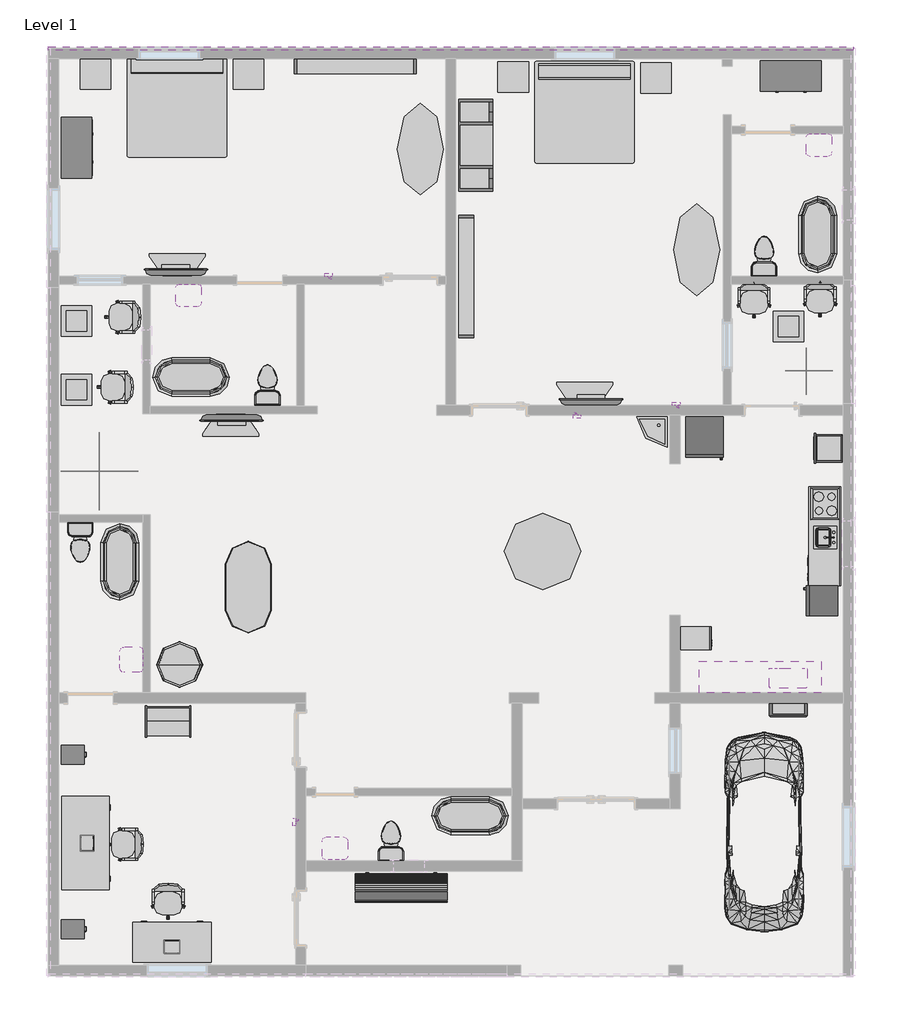
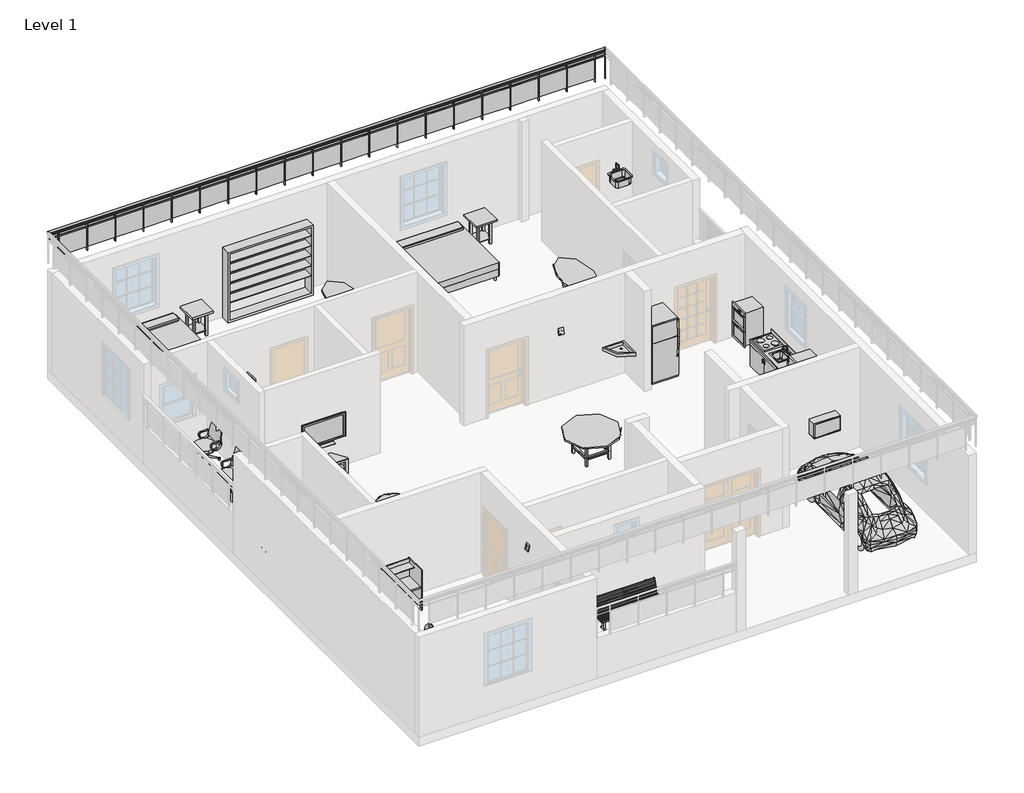
# One storey, part 4 of 4: 37 furniture elements, 17 proxies, 14 flow terminals, 3 geographic elements, 1 railing.
"""IFC4 building model written with IfcOpenShell, lengths in millimetres."""

from ifc_helpers import new_model, si_unit, point, frame, origin, place, context, project, spatial, polyline, ellipse_curve, trimmed, outline, extrude, transform, mapped, element, save
from ifc_brep_helpers import plane_surface, extruded_surface, advanced_brep
from components import entourage_4c8cfd20, proxy_7e1014cc, proxy_a6faaae8, proxy_45b28599, kitchenette_medium_kitchenette_medium_844211aa, proxy_8a8d5ab2, proxy_8b8c2dc4, rpc_beetle_rpc_beetle_3ce7ba48, rpc_picture_frame_rpc_picture_frame_c25e3fe9, proxy_c523a7b7, proxy_a13a33b2, single_carrel_single_carrel_ed4d160c, flow_terminal_bd5cdcf8, flow_terminal_871c2e40, flow_terminal_62a433f7, toilet_domestic_3d_toilet_domestic_3d_f7549cf7, toilet_domestic_3d_toilet_domestic_3d_183bbd19, flow_terminal_b374fae2, furniture_1fc5af50, furniture_d4d3357e, chair_executive_chair_executive_8d69e98c, furniture_22cae41e, furniture_c6510c7c, furniture_072f6425, furniture_2fc54265, furniture_9fa109b2, furniture_cf0b6580, furniture_b1da5ad0, furniture_fdf74506, tv_stand_tv_stand_6ce107e5, furniture_b5c51a22, furniture_2c34a4f9, furniture_bbcc68ce, furniture_027a2ad9, furniture_5bc9ed15, furniture_c80d6d9c, geographic_element_235d1464, geographic_element_ca6e1e19, geographic_element_e27c54a3

model = new_model("IFC4")

# Units and contexts
model_context = context("Model", 3, world=origin())
ifc_project = project(units=[si_unit("LENGTHUNIT", "METRE", prefix="MILLI")], contexts=[model_context])

# Site, building, storey
site = spatial("IfcSite", under=ifc_project)
building = spatial("IfcBuilding", under=site)
storey = spatial("IfcBuildingStorey", under=building, Name="Level 1", Elevation=0.0)

# Proxies
placement = place(None, origin())
entourage_shape = entourage_4c8cfd20(model_context)
element("IfcBuildingElementProxy", 1, Name="Entourage", at=placement, inside=storey, context=model_context, shape_type="MappedRepresentation", body=[
    mapped(entourage_shape, transform((-16905.1484731, -3276.9557719, 762.0), x_axis=(0.0, 1.0, 0.0), y_axis=(-1.0, 0.0, 0.0), z_axis=(0.0, 0.0, 1.0))),
])
element("IfcBuildingElementProxy", 2, Name="Entourage", at=placement, inside=storey, context=model_context, shape_type="MappedRepresentation", body=[
    mapped(entourage_shape, transform((-15177.9484731, -5385.1557719, 762.0), x_axis=(-1.0, 0.0, 0.0), y_axis=(0.0, -1.0, 0.0), z_axis=(0.0, 0.0, 1.0))),
])
proxy_shape = proxy_7e1014cc(model_context)
element("IfcBuildingElementProxy", 3, Name="18\" x 24\" x 34 1/2\"", ObjectType="18\" x 24\" x 34 1/2\"", at=placement, inside=storey, context=model_context, shape_type="MappedRepresentation", body=[
    mapped(proxy_shape, transform((-4472.0989083, 506.3267596, 0.0), x_axis=(0.0, 1.0, 0.0), y_axis=(-1.0, 0.0, 0.0), z_axis=(0.0, 0.0, 1.0))),
])
proxy_2_shape = proxy_a6faaae8(model_context)
element("IfcBuildingElementProxy", 4, Name="Cook Top-4 Unit2 : 22\" x 20\"", ObjectType="Cook Top-4 Unit2 : 22\" x 20\"", at=placement, inside=storey, context=model_context, shape_type="MappedRepresentation", body=[
    mapped(proxy_2_shape, transform((-2147.7484731, 3492.1442281, 0.0), x_axis=(0.0, -1.0, 0.0), y_axis=(1.0, 0.0, 0.0), z_axis=(0.0, 0.0, 1.0))),
])
proxy_3_shape = proxy_45b28599(model_context)
element("IfcBuildingElementProxy", 5, Name="Dishwasher : 24\" x 24\" x 34\"", ObjectType="Dishwasher : 24\" x 24\" x 34\"", at=placement, inside=storey, context=model_context, shape_type="MappedRepresentation", body=[
    mapped(proxy_3_shape, transform((-2439.5980379, 2540.9616966, 0.0), x_axis=(0.0, -1.0, 0.0), y_axis=(1.0, 0.0, 0.0), z_axis=(0.0, 0.0, 1.0))),
])
kitchenette_medium_kitchenette_medium_shape = kitchenette_medium_kitchenette_medium_844211aa(model_context)
element("IfcBuildingElementProxy", 6, Name="Kitchenette - Medium : Kitchenette - Medium", ObjectType="Kitchenette - Medium : Kitchenette - Medium", at=placement, inside=storey, context=model_context, shape_type="MappedRepresentation", body=[
    mapped(kitchenette_medium_kitchenette_medium_shape, transform((-1842.9484731, 3167.981933, 0.0), x_axis=(0.0, -1.0, 0.0), y_axis=(1.0, 0.0, 0.0), z_axis=(0.0, 0.0, 1.0))),
])
proxy_4_shape = proxy_8a8d5ab2(model_context)
element("IfcBuildingElementProxy", 7, Name="Microwave : 30\" x 16\" x 18\"", ObjectType="Microwave : 30\" x 16\" x 18\"", at=placement, inside=storey, context=model_context, shape_type="MappedRepresentation", body=[
    mapped(proxy_4_shape, transform((-2384.0555957, -912.2362777, 0.0), x_axis=(-1.0000000000000004, 0.0, 0.0), y_axis=(0.0, -1.0000000000000004, 0.0), z_axis=(0.0, 0.0, 1.0))),
])
element("IfcBuildingElementProxy", 8, Name="Microwave : 30\" x 16\" x 18\"", ObjectType="Microwave : 30\" x 16\" x 18\"", at=placement, inside=storey, context=model_context, shape_type="MappedRepresentation", body=[
    mapped(proxy_4_shape, transform((-2384.0555957, -340.7362777, 609.6), x_axis=(-1.0000000000000013, 0.0, 0.0), y_axis=(0.0, -1.0000000000000013, 0.0), z_axis=(0.0, 0.0, 1.0))),
])
proxy_5_shape = proxy_8b8c2dc4(model_context)
element("IfcBuildingElementProxy", 9, Name="Oven Double-Built-in : 21 1/2\" x 39 1/4\" x 21\"", ObjectType="Oven Double-Built-in : 21 1/2\" x 39 1/4\" x 21\"", at=placement, inside=storey, context=model_context, shape_type="MappedRepresentation", body=[
    mapped(proxy_5_shape, transform((-2212.614332, 4561.8693008, 0.0), x_axis=(0.0, -1.0000000000000004, 0.0), y_axis=(1.0000000000000004, 0.0, 0.0), z_axis=(0.0, 0.0, 1.0))),
])
rpc_beetle_rpc_beetle_shape = rpc_beetle_rpc_beetle_3ce7ba48(model_context)
element("IfcBuildingElementProxy", 10, Name="RPC Beetle : RPC Beetle", ObjectType="RPC Beetle : RPC Beetle", at=placement, inside=storey, context=model_context, shape_type="MappedRepresentation", body=[
    mapped(rpc_beetle_rpc_beetle_shape, transform((-3366.9484731, -4292.9557719, 0.0), x_axis=(1.0, 0.0, 0.0), y_axis=(0.0, 1.0, 0.0), z_axis=(0.0, 0.0, 1.0))),
])
rpc_picture_frame_rpc_picture_frame_shape = rpc_picture_frame_rpc_picture_frame_c25e3fe9(model_context)
element("IfcBuildingElementProxy", 11, Name="RPC Picture Frame : RPC Picture Frame", ObjectType="RPC Picture Frame : RPC Picture Frame", at=placement, inside=storey, context=model_context, shape_type="MappedRepresentation", body=[
    mapped(rpc_picture_frame_rpc_picture_frame_shape, transform((-12053.7484731, 8026.0442281, 1828.8), x_axis=(-1.0000000000000002, 0.0, 0.0), y_axis=(0.0, -1.0000000000000002, 0.0), z_axis=(0.0, 0.0, 1.0))),
])
element("IfcBuildingElementProxy", 12, Name="RPC Picture Frame : RPC Picture Frame", ObjectType="RPC Picture Frame : RPC Picture Frame", at=placement, inside=storey, context=model_context, shape_type="MappedRepresentation", body=[
    mapped(rpc_picture_frame_rpc_picture_frame_shape, transform((-5119.5484731, 5460.6442281, 1828.8), x_axis=(-1.0000000000000002, 0.0, 0.0), y_axis=(0.0, -1.0000000000000002, 0.0), z_axis=(0.0, 0.0, 1.0))),
])
element("IfcBuildingElementProxy", 13, Name="RPC Picture Frame : RPC Picture Frame", ObjectType="RPC Picture Frame : RPC Picture Frame", at=placement, inside=storey, context=model_context, shape_type="MappedRepresentation", body=[
    mapped(rpc_picture_frame_rpc_picture_frame_shape, transform((-7100.7484731, 5257.4442281, 1828.8), x_axis=(1.0, 0.0, 0.0), y_axis=(0.0, 1.0, 0.0), z_axis=(0.0, 0.0, 1.0))),
])
element("IfcBuildingElementProxy", 14, Name="RPC Picture Frame : RPC Picture Frame", ObjectType="RPC Picture Frame : RPC Picture Frame", at=placement, inside=storey, context=model_context, shape_type="MappedRepresentation", body=[
    mapped(rpc_picture_frame_rpc_picture_frame_shape, transform((-12714.1484731, -2857.8557719, 2133.6), x_axis=(0.0, -1.0, 0.0), y_axis=(1.0, 0.0, 0.0), z_axis=(0.0, 0.0, 1.0))),
])
proxy_6_shape = proxy_c523a7b7(model_context)
element("IfcBuildingElementProxy", 15, Name="Refrigerator : 24\" x 25\" LH", ObjectType="Refrigerator : 24\" x 25\" LH", at=placement, inside=storey, context=model_context, shape_type="MappedRepresentation", body=[
    mapped(proxy_6_shape, transform((-2193.3974446, 1555.3942281, 0.0), x_axis=(0.0, -1.0, 0.0), y_axis=(1.0, 0.0, 0.0), z_axis=(0.0, 0.0, 1.0))),
])
proxy_7_shape = proxy_a13a33b2(model_context)
element("IfcBuildingElementProxy", 16, Name="Refrigerator.0001 : 30\" x 32\" RH", ObjectType="Refrigerator.0001 : 30\" x 32\" RH", at=placement, inside=storey, context=model_context, shape_type="MappedRepresentation", body=[
    mapped(proxy_7_shape, transform((-4552.8109731, 4839.5431996, 0.0), x_axis=(1.0000000000000009, 0.0, 0.0), y_axis=(0.0, 1.0000000000000009, 0.0), z_axis=(0.0, 0.0, 1.0))),
])
single_carrel_single_carrel_shape = single_carrel_single_carrel_ed4d160c(model_context)
element("IfcBuildingElementProxy", 17, Name="Single Carrel : Single Carrel", ObjectType="Single Carrel : Single Carrel", at=placement, inside=storey, context=model_context, shape_type="MappedRepresentation", body=[
    mapped(single_carrel_single_carrel_shape, transform((-15254.1484731, -559.1557719, 0.0), x_axis=(1.0, 0.0, 0.0), y_axis=(0.0, 1.0, 0.0), z_axis=(0.0, 0.0, 1.0))),
])

# Flow terminals
flow_terminal_shape = flow_terminal_bd5cdcf8(model_context)
element("IfcFlowTerminal", 18, ObjectType="Sink - Corner Floor : 24\"", at=placement, inside=storey, context=model_context, shape_type="MappedRepresentation", body=[
    mapped(flow_terminal_shape, transform((-5297.3484731, 5232.0442281, 914.4), x_axis=(-1.0000000000000002, 0.0, 0.0), y_axis=(0.0, -1.0000000000000002, 0.0), z_axis=(0.0, 0.0, 1.0))),
])
flow_terminal_2_shape = flow_terminal_871c2e40(model_context)
element("IfcFlowTerminal", 19, ObjectType="Sink Kitchen-Island : 18\" x 18\"", at=placement, inside=storey, context=model_context, shape_type="MappedRepresentation", body=[
    mapped(flow_terminal_2_shape, transform((-2150.0938742, 2834.7334687, -14.4), x_axis=(0.0, -1.0, 0.0), y_axis=(1.0, 0.0, 0.0), z_axis=(0.0, 0.0, 1.0))),
])
flow_terminal_3_shape = flow_terminal_62a433f7(model_context)
element("IfcFlowTerminal", 20, ObjectType="Sink Vanity-Square : 20\" x 18\"", at=placement, inside=storey, context=model_context, shape_type="MappedRepresentation", body=[
    mapped(flow_terminal_3_shape, transform((-14863.4377136, 7693.498827, 914.4), x_axis=(1.0, 0.0, 0.0), y_axis=(0.0, 1.0, 0.0), z_axis=(0.0, 0.0, 1.0))),
])
element("IfcFlowTerminal", 21, ObjectType="Sink Vanity-Square : 20\" x 18\"", at=placement, inside=storey, context=model_context, shape_type="MappedRepresentation", body=[
    mapped(flow_terminal_3_shape, transform((-2290.4377136, 10690.698827, 914.4), x_axis=(1.0, 0.0, 0.0), y_axis=(0.0, 1.0, 0.0), z_axis=(0.0, 0.0, 1.0))),
])
element("IfcFlowTerminal", 22, ObjectType="Sink Vanity-Square : 20\" x 18\"", at=placement, inside=storey, context=model_context, shape_type="MappedRepresentation", body=[
    mapped(flow_terminal_3_shape, transform((-15942.2938742, 396.3334687, 914.4), x_axis=(0.0, -1.0000000000000004, 0.0), y_axis=(1.0000000000000004, 0.0, 0.0), z_axis=(0.0, 0.0, 1.0))),
])
element("IfcFlowTerminal", 23, ObjectType="Sink Vanity-Square : 20\" x 18\"", at=placement, inside=storey, context=model_context, shape_type="MappedRepresentation", body=[
    mapped(flow_terminal_3_shape, transform((-11911.0592325, -3427.0103708, 914.4), x_axis=(-1.0, 0.0, 0.0), y_axis=(0.0, -1.0, 0.0), z_axis=(0.0, 0.0, 1.0))),
])
toilet_domestic_3d_toilet_domestic_3d_shape = toilet_domestic_3d_toilet_domestic_3d_f7549cf7(model_context)
toilet_domestic_3d_toilet_domestic_3d_2_shape = toilet_domestic_3d_toilet_domestic_3d_183bbd19(model_context)
element("IfcFlowTerminal", 24, ObjectType="Toilet-Domestic-3D : Toilet-Domestic-3D", at=placement, inside=storey, context=model_context, shape_type="MappedRepresentation", body=[
    mapped(toilet_domestic_3d_toilet_domestic_3d_shape, transform((-13272.9484731, 5955.3402555, 0.0), x_axis=(-1.0, 0.0, 0.0), y_axis=(0.0, -1.0, 0.0), z_axis=(0.0, 0.0, 1.0))),
    mapped(toilet_domestic_3d_toilet_domestic_3d_2_shape, transform((-13272.9484731, 5955.3402555, 0.0), x_axis=(-1.0, 0.0, 0.0), y_axis=(0.0, -1.0, 0.0), z_axis=(0.0, 0.0, 1.0))),
])
element("IfcFlowTerminal", 25, ObjectType="Toilet-Domestic-3D : Toilet-Domestic-3D", at=placement, inside=storey, context=model_context, shape_type="MappedRepresentation", body=[
    mapped(toilet_domestic_3d_toilet_domestic_3d_shape, transform((-3366.9484731, 8520.7402555, 0.0), x_axis=(-1.0, 0.0, 0.0), y_axis=(0.0, -1.0, 0.0), z_axis=(0.0, 0.0, 1.0))),
    mapped(toilet_domestic_3d_toilet_domestic_3d_2_shape, transform((-3366.9484731, 8520.7402555, 0.0), x_axis=(-1.0, 0.0, 0.0), y_axis=(0.0, -1.0, 0.0), z_axis=(0.0, 0.0, 1.0))),
])
element("IfcFlowTerminal", 26, ObjectType="Toilet-Domestic-3D : Toilet-Domestic-3D", at=placement, inside=storey, context=model_context, shape_type="MappedRepresentation", body=[
    mapped(toilet_domestic_3d_toilet_domestic_3d_shape, transform((-17006.7484731, 2629.1482008, 0.0), x_axis=(1.0, 0.0, 0.0), y_axis=(0.0, 1.0, 0.0), z_axis=(0.0, 0.0, 1.0))),
    mapped(toilet_domestic_3d_toilet_domestic_3d_2_shape, transform((-17006.7484731, 2629.1482008, 0.0), x_axis=(1.0, 0.0, 0.0), y_axis=(0.0, 1.0, 0.0), z_axis=(0.0, 0.0, 1.0))),
])
element("IfcFlowTerminal", 27, ObjectType="Toilet-Domestic-3D : Toilet-Domestic-3D", at=placement, inside=storey, context=model_context, shape_type="MappedRepresentation", body=[
    mapped(toilet_domestic_3d_toilet_domestic_3d_shape, transform((-10809.7524457, -3143.3728146, 0.0), x_axis=(-1.0, 0.0, 0.0), y_axis=(0.0, -1.0, 0.0), z_axis=(0.0, 0.0, 1.0))),
    mapped(toilet_domestic_3d_toilet_domestic_3d_2_shape, transform((-10809.7524457, -3143.3728146, 0.0), x_axis=(-1.0, 0.0, 0.0), y_axis=(0.0, -1.0, 0.0), z_axis=(0.0, 0.0, 1.0))),
])
flow_terminal_4_shape = flow_terminal_b374fae2(model_context)
element("IfcFlowTerminal", 28, ObjectType="Tub-Free Standing-3D : 30\" x 60\"", at=placement, inside=storey, context=model_context, shape_type="MappedRepresentation", body=[
    mapped(flow_terminal_4_shape, transform((-2300.1484731, 8864.2442281, 0.0), x_axis=(-1.0000000000000002, 0.0, 0.0), y_axis=(0.0, -1.0000000000000002, 0.0), z_axis=(0.0, 0.0, 1.0))),
])
element("IfcFlowTerminal", 29, ObjectType="Tub-Free Standing-3D : 30\" x 60\"", at=placement, inside=storey, context=model_context, shape_type="MappedRepresentation", body=[
    mapped(flow_terminal_4_shape, transform((-14796.9484731, 6019.4442281, 0.0), x_axis=(0.0, 1.0000000000000004, 0.0), y_axis=(-1.0000000000000004, 0.0, 0.0), z_axis=(0.0, 0.0, 1.0))),
])
element("IfcFlowTerminal", 30, ObjectType="Tub-Free Standing-3D : 30\" x 60\"", at=placement, inside=storey, context=model_context, shape_type="MappedRepresentation", body=[
    mapped(flow_terminal_4_shape, transform((-16219.3484731, 2330.6431503, 0.0), x_axis=(1.0000000000000002, 0.0, 0.0), y_axis=(0.0, 1.0000000000000002, 0.0), z_axis=(0.0, 0.0, 1.0))),
])
element("IfcFlowTerminal", 31, ObjectType="Tub-Free Standing-3D : 30\" x 60\"", at=placement, inside=storey, context=model_context, shape_type="MappedRepresentation", body=[
    mapped(flow_terminal_4_shape, transform((-9234.3484731, -2733.7411816, 0.0), x_axis=(0.0, -1.0000000000000004, 0.0), y_axis=(1.0000000000000004, 0.0, 0.0), z_axis=(0.0, 0.0, 1.0))),
])

# Furniture
furniture_shape = furniture_1fc5af50(model_context)
element("IfcFurniture", 32, ObjectType="Bed-Standard.0001 : King 78\" x 80\"", at=placement, inside=storey, context=model_context, shape_type="MappedRepresentation", body=[
    mapped(furniture_shape, transform((-15347.8369977, 11462.5393101, 0.0), x_axis=(1.0, 0.0, 0.0), y_axis=(0.0, 1.0, 0.0), z_axis=(0.0, 0.0, 1.0))),
])
element("IfcFurniture", 33, ObjectType="Bed-Standard.0001 : King 78\" x 80\"", at=placement, inside=storey, context=model_context, shape_type="MappedRepresentation", body=[
    mapped(furniture_shape, transform((-7219.8369977, 11348.2393101, 0.0), x_axis=(1.0, 0.0, 0.0), y_axis=(0.0, 1.0, 0.0), z_axis=(0.0, 0.0, 1.0))),
])
furniture_2_shape = furniture_d4d3357e(model_context)
element("IfcFurniture", 34, ObjectType="Cabinet-File 5 Drawer : 15\" x 18\"", at=placement, inside=storey, context=model_context, shape_type="MappedRepresentation", body=[
    mapped(furniture_2_shape, transform((-17301.2827732, -4863.5593248, 0.0), x_axis=(0.0, 1.0, 0.0), y_axis=(-1.0, 0.0, 0.0), z_axis=(0.0, 0.0, 1.0))),
])
element("IfcFurniture", 35, ObjectType="Cabinet-File 5 Drawer : 15\" x 18\"", at=placement, inside=storey, context=model_context, shape_type="MappedRepresentation", body=[
    mapped(furniture_2_shape, transform((-17301.2827732, -1383.7593248, 0.0), x_axis=(0.0, 1.0, 0.0), y_axis=(-1.0, 0.0, 0.0), z_axis=(0.0, 0.0, 1.0))),
])
chair_executive_chair_executive_shape = chair_executive_chair_executive_8d69e98c(model_context)
element("IfcFurniture", 36, ObjectType="Chair-Executive : Chair-Executive", at=placement, inside=storey, context=model_context, shape_type="MappedRepresentation", body=[
    mapped(chair_executive_chair_executive_shape, transform((-16149.6025714, 7072.2534084, 0.0), x_axis=(0.0, 1.0, 0.0), y_axis=(-1.0, 0.0, 0.0), z_axis=(0.0, 0.0, 1.0))),
])
element("IfcFurniture", 37, ObjectType="Chair-Executive : Chair-Executive", at=placement, inside=storey, context=model_context, shape_type="MappedRepresentation", body=[
    mapped(chair_executive_chair_executive_shape, transform((-16302.0025714, 5675.2534084, 0.0), x_axis=(0.0, 1.0, 0.0), y_axis=(-1.0, 0.0, 0.0), z_axis=(0.0, 0.0, 1.0))),
])
element("IfcFurniture", 38, ObjectType="Chair-Executive : Chair-Executive", at=placement, inside=storey, context=model_context, shape_type="MappedRepresentation", body=[
    mapped(chair_executive_chair_executive_shape, transform((-3429.1576534, 7562.3901298, 0.0), x_axis=(-1.0000000000000018, 0.0, 0.0), y_axis=(0.0, -1.0000000000000018, 0.0), z_axis=(0.0, 0.0, 1.0))),
])
element("IfcFurniture", 39, ObjectType="Chair-Executive : Chair-Executive", at=placement, inside=storey, context=model_context, shape_type="MappedRepresentation", body=[
    mapped(chair_executive_chair_executive_shape, transform((-2108.3576534, 7587.7901298, 0.0), x_axis=(-1.0000000000000002, 0.0, 0.0), y_axis=(0.0, -1.0000000000000002, 0.0), z_axis=(0.0, 0.0, 1.0))),
])
element("IfcFurniture", 40, ObjectType="Chair-Executive : Chair-Executive", at=placement, inside=storey, context=model_context, shape_type="MappedRepresentation", body=[
    mapped(chair_executive_chair_executive_shape, transform((-16098.8025714, -3443.3465916, 0.0), x_axis=(0.0, 1.0, 0.0), y_axis=(-1.0, 0.0, 0.0), z_axis=(0.0, 0.0, 1.0))),
])
element("IfcFurniture", 41, ObjectType="Chair-Executive : Chair-Executive", at=placement, inside=storey, context=model_context, shape_type="MappedRepresentation", body=[
    mapped(chair_executive_chair_executive_shape, transform((-15113.1576534, -4426.4098702, 0.0), x_axis=(-1.0000000000000002, 0.0, 0.0), y_axis=(0.0, -1.0000000000000002, 0.0), z_axis=(0.0, 0.0, 1.0))),
])
furniture_3_shape = furniture_22cae41e(model_context)
element("IfcFurniture", 42, ObjectType="Counter Top w Sink Hole : 24\" Depth", at=placement, inside=storey, context=model_context, shape_type="MappedRepresentation", body=[
    mapped(furniture_3_shape, transform((-3461.886178, 355.2442281, 609.6), x_axis=(1.0, 0.0, 0.0), y_axis=(0.0, 1.0, 0.0), z_axis=(0.0, 0.0, 1.0))),
])
furniture_4_shape = furniture_c6510c7c(model_context)
element("IfcFurniture", 43, ObjectType="Counter Top w Sink Hole : 24\" Depth", at=placement, inside=storey, context=model_context, shape_type="MappedRepresentation", body=[
    mapped(furniture_4_shape, transform((-1842.9484731, 2634.581933, -14.4), x_axis=(0.0, -1.0, 0.0), y_axis=(1.0, 0.0, 0.0), z_axis=(0.0, 0.0, 1.0))),
])
furniture_5_shape = furniture_072f6425(model_context)
element("IfcFurniture", 44, ObjectType="Desk : 60\" x 30\" Student", at=placement, inside=storey, context=model_context, shape_type="MappedRepresentation", body=[
    mapped(furniture_5_shape, transform((-15939.9484731, -5639.1557719, 0.0), x_axis=(1.0, 0.0, 0.0), y_axis=(0.0, 1.0, 0.0), z_axis=(0.0, 0.0, 1.0))),
])
furniture_6_shape = furniture_2fc54265(model_context)
element("IfcFurniture", 45, ObjectType="Desk : 72\" x 36\"", at=placement, inside=storey, context=model_context, shape_type="MappedRepresentation", body=[
    mapped(furniture_6_shape, transform((-17362.3484731, -2362.5557719, 0.0), x_axis=(0.0, -1.0000000000000004, 0.0), y_axis=(1.0000000000000004, 0.0, 0.0), z_axis=(0.0, 0.0, 1.0))),
])
furniture_7_shape = furniture_9fa109b2(model_context)
element("IfcFurniture", 46, ObjectType="Dresser : 48\" x 72\" x 24\"", at=placement, inside=storey, context=model_context, shape_type="MappedRepresentation", body=[
    mapped(furniture_7_shape, transform((-17446.1114272, 10860.637488, 0.0), x_axis=(0.0, 1.0, 0.0), y_axis=(-1.0, 0.0, 0.0), z_axis=(0.0, 0.0, 1.0))),
])
element("IfcFurniture", 47, ObjectType="Dresser : 48\" x 72\" x 24\"", at=placement, inside=storey, context=model_context, shape_type="MappedRepresentation", body=[
    mapped(furniture_7_shape, transform((-2564.3552132, 12389.7071822, 0.0), x_axis=(1.0000000000000007, 0.0, 0.0), y_axis=(0.0, 1.0000000000000007, 0.0), z_axis=(0.0, 0.0, 1.0))),
])
furniture_8_shape = furniture_cf0b6580(model_context)
element("IfcFurniture", 48, ObjectType="Entertainment Center : 72\" x 72\" x 24\"", at=placement, inside=storey, context=model_context, shape_type="MappedRepresentation", body=[
    mapped(furniture_8_shape, transform((-9564.5484731, 10642.2442281, 0.0), x_axis=(0.0, 1.0, 0.0), y_axis=(-1.0, 0.0, 0.0), z_axis=(0.0, 0.0, 1.0))),
])
furniture_9_shape = furniture_b1da5ad0(model_context)
element("IfcFurniture", 49, ObjectType="Shelving : 96\" x 12\" x 84\"", at=placement, inside=storey, context=model_context, shape_type="MappedRepresentation", body=[
    mapped(furniture_9_shape, transform((-11520.3484731, 12521.8442281, 0.0), x_axis=(1.0, 0.0, 0.0), y_axis=(0.0, 1.0, 0.0), z_axis=(0.0, 0.0, 1.0))),
])
element("IfcFurniture", 50, ObjectType="Shelving : 96\" x 12\" x 84\"", at=placement, inside=storey, context=model_context, shape_type="MappedRepresentation", body=[
    mapped(furniture_9_shape, transform((-9615.3484731, 8026.0442281, 0.0), x_axis=(0.0, 1.0000000000000002, 0.0), y_axis=(-1.0000000000000002, 0.0, 0.0), z_axis=(0.0, 0.0, 1.0))),
])
furniture_10_shape = furniture_fdf74506(model_context)
element("IfcFurniture", 51, ObjectType="TV - Flat Screen : 50\"", at=placement, inside=storey, context=model_context, shape_type="MappedRepresentation", body=[
    mapped(furniture_10_shape, transform((-15105.6929872, 8105.4337019, 914.4), x_axis=(-1.0000000000000002, 0.0, 0.0), y_axis=(0.0, -1.0000000000000002, 0.0), z_axis=(0.0, 0.0, 1.0))),
])
element("IfcFurniture", 52, ObjectType="TV - Flat Screen : 50\"", at=placement, inside=storey, context=model_context, shape_type="MappedRepresentation", body=[
    mapped(furniture_10_shape, transform((-6825.2929872, 5519.1828518, 914.4), x_axis=(-1.0000000000000002, 0.0, 0.0), y_axis=(0.0, -1.0000000000000002, 0.0), z_axis=(0.0, 0.0, 1.0))),
])
element("IfcFurniture", 53, ObjectType="TV - Flat Screen : 50\"", at=placement, inside=storey, context=model_context, shape_type="MappedRepresentation", body=[
    mapped(furniture_10_shape, transform((-13982.5656994, 5210.6304677, 914.4), x_axis=(1.0000000000000007, 0.0, 0.0), y_axis=(0.0, 1.0000000000000007, 0.0), z_axis=(0.0, 0.0, 1.0))),
])
tv_stand_tv_stand_shape = tv_stand_tv_stand_6ce107e5(model_context)
element("IfcFurniture", 54, ObjectType="TV Stand : TV Stand", at=placement, inside=storey, context=model_context, shape_type="MappedRepresentation", body=[
    mapped(tv_stand_tv_stand_shape, transform((-14951.160471, 8026.0442281, 0.0), x_axis=(-1.0, 0.0, 0.0), y_axis=(0.0, -1.0, 0.0), z_axis=(0.0, 0.0, 1.0))),
])
element("IfcFurniture", 55, ObjectType="TV Stand : TV Stand", at=placement, inside=storey, context=model_context, shape_type="MappedRepresentation", body=[
    mapped(tv_stand_tv_stand_shape, transform((-6823.160471, 5460.6442281, 0.0), x_axis=(-1.0, 0.0, 0.0), y_axis=(0.0, -1.0, 0.0), z_axis=(0.0, 0.0, 1.0))),
])
element("IfcFurniture", 56, ObjectType="TV Stand : TV Stand", at=placement, inside=storey, context=model_context, shape_type="MappedRepresentation", body=[
    mapped(tv_stand_tv_stand_shape, transform((-14134.7364751, 5298.6986547, 0.0), x_axis=(1.0000000000000004, 0.0, 0.0), y_axis=(0.0, 1.0000000000000004, 0.0), z_axis=(0.0, 0.0, 1.0))),
])
furniture_11_shape = furniture_b5c51a22(model_context)
element("IfcFurniture", 57, ObjectType="Table-Coffee : 24\" x 24\" x 24\"", at=placement, inside=storey, context=model_context, shape_type="MappedRepresentation", body=[
    mapped(furniture_11_shape, transform((-17101.2142397, 5670.2331503, 0.0), x_axis=(1.0, 0.0, 0.0), y_axis=(0.0, 1.0, 0.0), z_axis=(0.0, 0.0, 1.0))),
])
element("IfcFurniture", 58, ObjectType="Table-Coffee : 24\" x 24\" x 24\"", at=placement, inside=storey, context=model_context, shape_type="MappedRepresentation", body=[
    mapped(furniture_11_shape, transform((-17101.2142397, 7041.8331503, 0.0), x_axis=(1.0, 0.0, 0.0), y_axis=(0.0, 1.0, 0.0), z_axis=(0.0, 0.0, 1.0))),
])
element("IfcFurniture", 59, ObjectType="Table-Coffee : 24\" x 24\" x 24\"", at=placement, inside=storey, context=model_context, shape_type="MappedRepresentation", body=[
    mapped(furniture_11_shape, transform((-2902.6142397, 6929.6370487, 0.0), x_axis=(1.0, 0.0, 0.0), y_axis=(0.0, 1.0, 0.0), z_axis=(0.0, 0.0, 1.0))),
])
furniture_12_shape = furniture_2c34a4f9(model_context)
element("IfcFurniture", 60, ObjectType="Table-Dining Oval : 36\" x 72\"", at=placement, inside=storey, context=model_context, shape_type="MappedRepresentation", body=[
    mapped(furniture_12_shape, transform((-14012.0468337, 2230.2639002, 0.0), x_axis=(0.0, 1.0, 0.0), y_axis=(-1.0, 0.0, 0.0), z_axis=(0.0, 0.0, 1.0))),
])
furniture_13_shape = furniture_bbcc68ce(model_context)
element("IfcFurniture", 61, ObjectType="Table-Dining Round w Chairs : 60\" Diameter", at=placement, inside=storey, context=model_context, shape_type="MappedRepresentation", body=[
    mapped(furniture_13_shape, transform((-7890.2304403, 2724.5229166, 0.0), x_axis=(1.0, 0.0, 0.0), y_axis=(0.0, 1.0, 0.0), z_axis=(0.0, 0.0, 1.0))),
])
furniture_14_shape = furniture_027a2ad9(model_context)
element("IfcFurniture", 62, ObjectType="Table-Ellipse : 72\" x 36\"", at=placement, inside=storey, context=model_context, shape_type="MappedRepresentation", body=[
    mapped(furniture_14_shape, transform((-10224.9484731, 10566.0442281, 0.0), x_axis=(0.0, 1.0, 0.0), y_axis=(-1.0, 0.0, 0.0), z_axis=(0.0, 0.0, 1.0))),
])
element("IfcFurniture", 63, ObjectType="Table-Ellipse : 72\" x 36\"", at=placement, inside=storey, context=model_context, shape_type="MappedRepresentation", body=[
    mapped(furniture_14_shape, transform((-4713.1484731, 8559.4442281, 0.0), x_axis=(0.0, -1.0000000000000007, 0.0), y_axis=(1.0000000000000007, 0.0, 0.0), z_axis=(0.0, 0.0, 1.0))),
])
furniture_15_shape = furniture_5bc9ed15(model_context)
element("IfcFurniture", 64, ObjectType="Table-Night Stand : 24\" x 24\" x 30\"", at=placement, inside=storey, context=model_context, shape_type="MappedRepresentation", body=[
    mapped(furniture_15_shape, transform((-17010.4821034, 11759.8442281, 0.0), x_axis=(1.0, 0.0, 0.0), y_axis=(0.0, 1.0, 0.0), z_axis=(0.0, 0.0, 1.0))),
])
element("IfcFurniture", 65, ObjectType="Table-Night Stand : 24\" x 24\" x 30\"", at=placement, inside=storey, context=model_context, shape_type="MappedRepresentation", body=[
    mapped(furniture_15_shape, transform((-13962.4821034, 11759.8442281, 0.0), x_axis=(1.0, 0.0, 0.0), y_axis=(0.0, 1.0, 0.0), z_axis=(0.0, 0.0, 1.0))),
])
element("IfcFurniture", 66, ObjectType="Table-Night Stand : 24\" x 24\" x 30\"", at=placement, inside=storey, context=model_context, shape_type="MappedRepresentation", body=[
    mapped(furniture_15_shape, transform((-8679.2821034, 11695.4815518, 0.0), x_axis=(1.0, 0.0, 0.0), y_axis=(0.0, 1.0, 0.0), z_axis=(0.0, 0.0, 1.0))),
])
element("IfcFurniture", 67, ObjectType="Table-Night Stand : 24\" x 24\" x 30\"", at=placement, inside=storey, context=model_context, shape_type="MappedRepresentation", body=[
    mapped(furniture_15_shape, transform((-5834.4821034, 11675.6602635, 0.0), x_axis=(1.0, 0.0, 0.0), y_axis=(0.0, 1.0, 0.0), z_axis=(0.0, 0.0, 1.0))),
])
furniture_16_shape = furniture_c80d6d9c(model_context)
element("IfcFurniture", 68, ObjectType="Table-Round : 36\" Diameter", at=placement, inside=storey, context=model_context, shape_type="MappedRepresentation", body=[
    mapped(furniture_16_shape, transform((-15025.5484731, 285.3942281, 0.0), x_axis=(1.0, 0.0, 0.0), y_axis=(0.0, 1.0, 0.0), z_axis=(0.0, 0.0, 1.0))),
])

# Geographic elements
geographic_element_shape = geographic_element_235d1464(model_context)
element("IfcGeographicElement", 69, ObjectType="Park Bench : 72\"", at=placement, inside=storey, context=model_context, shape_type="MappedRepresentation", body=[
    mapped(geographic_element_shape, transform((-10605.9484731, -4140.5557719, 0.0), x_axis=(1.0, 0.0, 0.0), y_axis=(0.0, 1.0, 0.0), z_axis=(0.0, 0.0, 1.0))),
])
geographic_element_2_shape = geographic_element_ca6e1e19(model_context)
element("IfcGeographicElement", 70, ObjectType="RPC Shrub : Burning Bush 4'-6\"", at=placement, inside=storey, context=model_context, shape_type="MappedRepresentation", body=[
    mapped(geographic_element_2_shape, transform((-16625.7484731, 4139.8442281, 0.0), x_axis=(1.0, 0.0, 0.0), y_axis=(0.0, 1.0, 0.0), z_axis=(0.0, 0.0, 1.0))),
])
geographic_element_3_shape = geographic_element_e27c54a3(model_context)
element("IfcGeographicElement", 71, ObjectType="RPC Shrub : Cedar Shrub 3'-0\"", at=placement, inside=storey, context=model_context, shape_type="MappedRepresentation", body=[
    mapped(geographic_element_3_shape, transform((-2528.7484731, 6146.4442281, 0.0), x_axis=(1.0, 0.0, 0.0), y_axis=(0.0, 1.0, 0.0), z_axis=(0.0, 0.0, 1.0))),
])

# Railing
element("IfcRailing", 72, ObjectType="Glass Panel - Bottom Fill", at=placement, inside=storey, context=model_context, shape_type="SolidModel", body=[
    advanced_brep(
    [(-17641.7484731, 12610.7442281, 4165.6), (-17641.7484731, 12534.5442281, 4165.6), (-1588.9484731, 12610.7442281, 4165.6), (-1588.9484731, 12534.5442281, 4165.6)],
    [
        (0, 1, ellipse_curve(frame((-17641.7484731, 12572.6442281, 4165.6), z_axis=(-1.0, 0.0, 0.0), x_axis=(0.0, -1.0, 0.0)), 38.1, 28.575)),
        (1, 0, ellipse_curve(frame((-17641.7484731, 12572.6442281, 4165.6), z_axis=(-1.0, 0.0, 0.0), x_axis=(0.0, -1.0, 0.0)), 38.1, 28.575)),
        (2, 3, ellipse_curve(frame((-1588.9484731, 12572.6442281, 4165.6), z_axis=(1.0, 0.0, 0.0), x_axis=(0.0, -1.0, 0.0)), 38.1, 28.575)),
        (3, 2, ellipse_curve(frame((-1588.9484731, 12572.6442281, 4165.6), z_axis=(1.0, 0.0, 0.0), x_axis=(0.0, -1.0, 0.0)), 38.1, 28.575)),
        (0, 2),
        (3, 1),
    ],
    [
        plane_surface(frame((-17641.7484731, 12572.6442281, 4165.6), z_axis=(-1.0, 0.0, 0.0), x_axis=(0.0, 1.0, 0.0))),
        plane_surface(frame((-1588.9484731, 12572.6442281, 4165.6), z_axis=(1.0, 0.0, 0.0), x_axis=(0.0, 1.0, 0.0))),
        extruded_surface(trimmed(ellipse_curve(frame((-1588.9484731, 12572.6442281, 4165.6), z_axis=(-1.0, 0.0, 0.0), x_axis=(0.0, -1.0, 0.0)), 38.1, 28.575), [point((-1588.9484731, 12610.7442281, 4165.6))], [point((-1588.9484731, 12534.5442281, 4165.6))], True, "CARTESIAN"), (-16052.800000000001, 0.0, 0.0), 16052.800000000001),
        extruded_surface(trimmed(ellipse_curve(frame((-1588.9484731, 12572.6442281, 4165.6), z_axis=(-1.0, 0.0, 0.0), x_axis=(0.0, -1.0, 0.0)), 38.1, 28.575), [point((-1588.9484731, 12534.5442281, 4165.6))], [point((-1588.9484731, 12610.7442281, 4165.6))], True, "CARTESIAN"), (-16052.800000000001, 0.0, 0.0), 16052.800000000001),
    ],
    [
        (0, [[1, 2]]),
        (1, [[3, 4]]),
        (2, [[-1, 5, -4, 6]]),
        (3, [[-2, -6, -3, -5]]),
    ],
),
    extrude(outline(polyline([(-17641.7484731, 12559.9442281), (-17641.7484731, 12585.3442281), (-1588.9484731, 12585.3442281), (-1588.9484731, 12559.9442281), (-17641.7484731, 12559.9442281)])), frame((0.0, 0.0, 4051.3), z_axis=(0.0, 0.0, 1.0), x_axis=(1.0, 0.0, 0.0)), (0.0, 0.0, 1.0), 25.4),
    extrude(outline(polyline([(-17641.7484731, 12559.9442281), (-17641.7484731, 12585.3442281), (-1588.9484731, 12585.3442281), (-1588.9484731, 12559.9442281), (-17641.7484731, 12559.9442281)])), frame((0.0, 0.0, 3949.7), z_axis=(0.0, 0.0, 1.0), x_axis=(1.0, 0.0, 0.0)), (0.0, 0.0, 1.0), 25.4),
    extrude(outline(polyline([(-1900.0984731, 12547.2442281), (-1900.0984731, 12598.0442281), (-1887.3984731, 12598.0442281), (-1887.3984731, 12547.2442281), (-1900.0984731, 12547.2442281)])), frame((0.0, 0.0, 3251.2), z_axis=(0.0, 0.0, 1.0), x_axis=(1.0, 0.0, 0.0)), (0.0, 0.0, 1.0), 885.6788223),
    extrude(outline(polyline([(-2706.5484731, 12579.1793851), (-1893.7484731, 12579.1793851), (-1893.7484731, 12572.8293851), (-2706.5484731, 12572.8293851), (-2706.5484731, 12579.1793851)])), frame((0.0, 0.0, 3352.8), z_axis=(0.0, 0.0, 1.0), x_axis=(1.0, 0.0, 0.0)), (0.0, 0.0, 1.0), 596.9),
    extrude(outline(polyline([(-2712.8984731, 12547.2442281), (-2712.8984731, 12598.0442281), (-2700.1984731, 12598.0442281), (-2700.1984731, 12547.2442281), (-2712.8984731, 12547.2442281)])), frame((0.0, 0.0, 3251.2), z_axis=(0.0, 0.0, 1.0), x_axis=(1.0, 0.0, 0.0)), (0.0, 0.0, 1.0), 885.6788223),
    extrude(outline(polyline([(-3519.3484731, 12579.1793851), (-2706.5484731, 12579.1793851), (-2706.5484731, 12572.8293851), (-3519.3484731, 12572.8293851), (-3519.3484731, 12579.1793851)])), frame((0.0, 0.0, 3352.8), z_axis=(0.0, 0.0, 1.0), x_axis=(1.0, 0.0, 0.0)), (0.0, 0.0, 1.0), 596.9),
    extrude(outline(polyline([(-3525.6984731, 12547.2442281), (-3525.6984731, 12598.0442281), (-3512.9984731, 12598.0442281), (-3512.9984731, 12547.2442281), (-3525.6984731, 12547.2442281)])), frame((0.0, 0.0, 3251.2), z_axis=(0.0, 0.0, 1.0), x_axis=(1.0, 0.0, 0.0)), (0.0, 0.0, 1.0), 885.6788223),
    extrude(outline(polyline([(-4332.1484731, 12579.1793851), (-3519.3484731, 12579.1793851), (-3519.3484731, 12572.8293851), (-4332.1484731, 12572.8293851), (-4332.1484731, 12579.1793851)])), frame((0.0, 0.0, 3352.8), z_axis=(0.0, 0.0, 1.0), x_axis=(1.0, 0.0, 0.0)), (0.0, 0.0, 1.0), 596.9),
    extrude(outline(polyline([(-4338.4984731, 12547.2442281), (-4338.4984731, 12598.0442281), (-4325.7984731, 12598.0442281), (-4325.7984731, 12547.2442281), (-4338.4984731, 12547.2442281)])), frame((0.0, 0.0, 3251.2), z_axis=(0.0, 0.0, 1.0), x_axis=(1.0, 0.0, 0.0)), (0.0, 0.0, 1.0), 885.6788223),
    extrude(outline(polyline([(-5144.9484731, 12579.1793851), (-4332.1484731, 12579.1793851), (-4332.1484731, 12572.8293851), (-5144.9484731, 12572.8293851), (-5144.9484731, 12579.1793851)])), frame((0.0, 0.0, 3352.8), z_axis=(0.0, 0.0, 1.0), x_axis=(1.0, 0.0, 0.0)), (0.0, 0.0, 1.0), 596.9),
    extrude(outline(polyline([(-5151.2984731, 12547.2442281), (-5151.2984731, 12598.0442281), (-5138.5984731, 12598.0442281), (-5138.5984731, 12547.2442281), (-5151.2984731, 12547.2442281)])), frame((0.0, 0.0, 3251.2), z_axis=(0.0, 0.0, 1.0), x_axis=(1.0, 0.0, 0.0)), (0.0, 0.0, 1.0), 885.6788223),
    extrude(outline(polyline([(-5957.7484731, 12579.1793851), (-5144.9484731, 12579.1793851), (-5144.9484731, 12572.8293851), (-5957.7484731, 12572.8293851), (-5957.7484731, 12579.1793851)])), frame((0.0, 0.0, 3352.8), z_axis=(0.0, 0.0, 1.0), x_axis=(1.0, 0.0, 0.0)), (0.0, 0.0, 1.0), 596.9),
    extrude(outline(polyline([(-5964.0984731, 12547.2442281), (-5964.0984731, 12598.0442281), (-5951.3984731, 12598.0442281), (-5951.3984731, 12547.2442281), (-5964.0984731, 12547.2442281)])), frame((0.0, 0.0, 3251.2), z_axis=(0.0, 0.0, 1.0), x_axis=(1.0, 0.0, 0.0)), (0.0, 0.0, 1.0), 885.6788223),
    extrude(outline(polyline([(-6770.5484731, 12579.1793851), (-5957.7484731, 12579.1793851), (-5957.7484731, 12572.8293851), (-6770.5484731, 12572.8293851), (-6770.5484731, 12579.1793851)])), frame((0.0, 0.0, 3352.8), z_axis=(0.0, 0.0, 1.0), x_axis=(1.0, 0.0, 0.0)), (0.0, 0.0, 1.0), 596.9),
    extrude(outline(polyline([(-6776.8984731, 12547.2442281), (-6776.8984731, 12598.0442281), (-6764.1984731, 12598.0442281), (-6764.1984731, 12547.2442281), (-6776.8984731, 12547.2442281)])), frame((0.0, 0.0, 3251.2), z_axis=(0.0, 0.0, 1.0), x_axis=(1.0, 0.0, 0.0)), (0.0, 0.0, 1.0), 885.6788223),
    extrude(outline(polyline([(-7583.3484731, 12579.1793851), (-6770.5484731, 12579.1793851), (-6770.5484731, 12572.8293851), (-7583.3484731, 12572.8293851), (-7583.3484731, 12579.1793851)])), frame((0.0, 0.0, 3352.8), z_axis=(0.0, 0.0, 1.0), x_axis=(1.0, 0.0, 0.0)), (0.0, 0.0, 1.0), 596.9),
    extrude(outline(polyline([(-7589.6984731, 12547.2442281), (-7589.6984731, 12598.0442281), (-7576.9984731, 12598.0442281), (-7576.9984731, 12547.2442281), (-7589.6984731, 12547.2442281)])), frame((0.0, 0.0, 3251.2), z_axis=(0.0, 0.0, 1.0), x_axis=(1.0, 0.0, 0.0)), (0.0, 0.0, 1.0), 885.6788223),
    extrude(outline(polyline([(-8396.1484731, 12579.1793851), (-7583.3484731, 12579.1793851), (-7583.3484731, 12572.8293851), (-8396.1484731, 12572.8293851), (-8396.1484731, 12579.1793851)])), frame((0.0, 0.0, 3352.8), z_axis=(0.0, 0.0, 1.0), x_axis=(1.0, 0.0, 0.0)), (0.0, 0.0, 1.0), 596.9),
    extrude(outline(polyline([(-8402.4984731, 12547.2442281), (-8402.4984731, 12598.0442281), (-8389.7984731, 12598.0442281), (-8389.7984731, 12547.2442281), (-8402.4984731, 12547.2442281)])), frame((0.0, 0.0, 3251.2), z_axis=(0.0, 0.0, 1.0), x_axis=(1.0, 0.0, 0.0)), (0.0, 0.0, 1.0), 885.6788223),
    extrude(outline(polyline([(-9208.9484731, 12579.1793851), (-8396.1484731, 12579.1793851), (-8396.1484731, 12572.8293851), (-9208.9484731, 12572.8293851), (-9208.9484731, 12579.1793851)])), frame((0.0, 0.0, 3352.8), z_axis=(0.0, 0.0, 1.0), x_axis=(1.0, 0.0, 0.0)), (0.0, 0.0, 1.0), 596.9),
    extrude(outline(polyline([(-9215.2984731, 12547.2442281), (-9215.2984731, 12598.0442281), (-9202.5984731, 12598.0442281), (-9202.5984731, 12547.2442281), (-9215.2984731, 12547.2442281)])), frame((0.0, 0.0, 3251.2), z_axis=(0.0, 0.0, 1.0), x_axis=(1.0, 0.0, 0.0)), (0.0, 0.0, 1.0), 885.6788223),
    extrude(outline(polyline([(-10021.7484731, 12579.1793851), (-9208.9484731, 12579.1793851), (-9208.9484731, 12572.8293851), (-10021.7484731, 12572.8293851), (-10021.7484731, 12579.1793851)])), frame((0.0, 0.0, 3352.8), z_axis=(0.0, 0.0, 1.0), x_axis=(1.0, 0.0, 0.0)), (0.0, 0.0, 1.0), 596.9),
    extrude(outline(polyline([(-10028.0984731, 12547.2442281), (-10028.0984731, 12598.0442281), (-10015.3984731, 12598.0442281), (-10015.3984731, 12547.2442281), (-10028.0984731, 12547.2442281)])), frame((0.0, 0.0, 3251.2), z_axis=(0.0, 0.0, 1.0), x_axis=(1.0, 0.0, 0.0)), (0.0, 0.0, 1.0), 885.6788223),
    extrude(outline(polyline([(-10834.5484731, 12579.1793851), (-10021.7484731, 12579.1793851), (-10021.7484731, 12572.8293851), (-10834.5484731, 12572.8293851), (-10834.5484731, 12579.1793851)])), frame((0.0, 0.0, 3352.8), z_axis=(0.0, 0.0, 1.0), x_axis=(1.0, 0.0, 0.0)), (0.0, 0.0, 1.0), 596.9),
    extrude(outline(polyline([(-10840.8984731, 12547.2442281), (-10840.8984731, 12598.0442281), (-10828.1984731, 12598.0442281), (-10828.1984731, 12547.2442281), (-10840.8984731, 12547.2442281)])), frame((0.0, 0.0, 3251.2), z_axis=(0.0, 0.0, 1.0), x_axis=(1.0, 0.0, 0.0)), (0.0, 0.0, 1.0), 885.6788223),
    extrude(outline(polyline([(-11647.3484731, 12579.1793851), (-10834.5484731, 12579.1793851), (-10834.5484731, 12572.8293851), (-11647.3484731, 12572.8293851), (-11647.3484731, 12579.1793851)])), frame((0.0, 0.0, 3352.8), z_axis=(0.0, 0.0, 1.0), x_axis=(1.0, 0.0, 0.0)), (0.0, 0.0, 1.0), 596.9),
    extrude(outline(polyline([(-11653.6984731, 12547.2442281), (-11653.6984731, 12598.0442281), (-11640.9984731, 12598.0442281), (-11640.9984731, 12547.2442281), (-11653.6984731, 12547.2442281)])), frame((0.0, 0.0, 3251.2), z_axis=(0.0, 0.0, 1.0), x_axis=(1.0, 0.0, 0.0)), (0.0, 0.0, 1.0), 885.6788223),
    extrude(outline(polyline([(-12460.1484731, 12579.1793851), (-11647.3484731, 12579.1793851), (-11647.3484731, 12572.8293851), (-12460.1484731, 12572.8293851), (-12460.1484731, 12579.1793851)])), frame((0.0, 0.0, 3352.8), z_axis=(0.0, 0.0, 1.0), x_axis=(1.0, 0.0, 0.0)), (0.0, 0.0, 1.0), 596.9),
    extrude(outline(polyline([(-12466.4984731, 12547.2442281), (-12466.4984731, 12598.0442281), (-12453.7984731, 12598.0442281), (-12453.7984731, 12547.2442281), (-12466.4984731, 12547.2442281)])), frame((0.0, 0.0, 3251.2), z_axis=(0.0, 0.0, 1.0), x_axis=(1.0, 0.0, 0.0)), (0.0, 0.0, 1.0), 885.6788223),
    extrude(outline(polyline([(-13272.9484731, 12579.1793851), (-12460.1484731, 12579.1793851), (-12460.1484731, 12572.8293851), (-13272.9484731, 12572.8293851), (-13272.9484731, 12579.1793851)])), frame((0.0, 0.0, 3352.8), z_axis=(0.0, 0.0, 1.0), x_axis=(1.0, 0.0, 0.0)), (0.0, 0.0, 1.0), 596.9),
    extrude(outline(polyline([(-13279.2984731, 12547.2442281), (-13279.2984731, 12598.0442281), (-13266.5984731, 12598.0442281), (-13266.5984731, 12547.2442281), (-13279.2984731, 12547.2442281)])), frame((0.0, 0.0, 3251.2), z_axis=(0.0, 0.0, 1.0), x_axis=(1.0, 0.0, 0.0)), (0.0, 0.0, 1.0), 885.6788223),
    extrude(outline(polyline([(-14085.7484731, 12579.1793851), (-13272.9484731, 12579.1793851), (-13272.9484731, 12572.8293851), (-14085.7484731, 12572.8293851), (-14085.7484731, 12579.1793851)])), frame((0.0, 0.0, 3352.8), z_axis=(0.0, 0.0, 1.0), x_axis=(1.0, 0.0, 0.0)), (0.0, 0.0, 1.0), 596.9),
    extrude(outline(polyline([(-14092.0984731, 12547.2442281), (-14092.0984731, 12598.0442281), (-14079.3984731, 12598.0442281), (-14079.3984731, 12547.2442281), (-14092.0984731, 12547.2442281)])), frame((0.0, 0.0, 3251.2), z_axis=(0.0, 0.0, 1.0), x_axis=(1.0, 0.0, 0.0)), (0.0, 0.0, 1.0), 885.6788223),
    extrude(outline(polyline([(-14898.5484731, 12579.1793851), (-14085.7484731, 12579.1793851), (-14085.7484731, 12572.8293851), (-14898.5484731, 12572.8293851), (-14898.5484731, 12579.1793851)])), frame((0.0, 0.0, 3352.8), z_axis=(0.0, 0.0, 1.0), x_axis=(1.0, 0.0, 0.0)), (0.0, 0.0, 1.0), 596.9),
    extrude(outline(polyline([(-14904.8984731, 12547.2442281), (-14904.8984731, 12598.0442281), (-14892.1984731, 12598.0442281), (-14892.1984731, 12547.2442281), (-14904.8984731, 12547.2442281)])), frame((0.0, 0.0, 3251.2), z_axis=(0.0, 0.0, 1.0), x_axis=(1.0, 0.0, 0.0)), (0.0, 0.0, 1.0), 885.6788223),
    extrude(outline(polyline([(-15711.3484731, 12579.1793851), (-14898.5484731, 12579.1793851), (-14898.5484731, 12572.8293851), (-15711.3484731, 12572.8293851), (-15711.3484731, 12579.1793851)])), frame((0.0, 0.0, 3352.8), z_axis=(0.0, 0.0, 1.0), x_axis=(1.0, 0.0, 0.0)), (0.0, 0.0, 1.0), 596.9),
    extrude(outline(polyline([(-15717.6984731, 12547.2442281), (-15717.6984731, 12598.0442281), (-15704.9984731, 12598.0442281), (-15704.9984731, 12547.2442281), (-15717.6984731, 12547.2442281)])), frame((0.0, 0.0, 3251.2), z_axis=(0.0, 0.0, 1.0), x_axis=(1.0, 0.0, 0.0)), (0.0, 0.0, 1.0), 885.6788223),
    extrude(outline(polyline([(-16524.1484731, 12579.1793851), (-15711.3484731, 12579.1793851), (-15711.3484731, 12572.8293851), (-16524.1484731, 12572.8293851), (-16524.1484731, 12579.1793851)])), frame((0.0, 0.0, 3352.8), z_axis=(0.0, 0.0, 1.0), x_axis=(1.0, 0.0, 0.0)), (0.0, 0.0, 1.0), 596.9),
    extrude(outline(polyline([(-16530.4984731, 12547.2442281), (-16530.4984731, 12598.0442281), (-16517.7984731, 12598.0442281), (-16517.7984731, 12547.2442281), (-16530.4984731, 12547.2442281)])), frame((0.0, 0.0, 3251.2), z_axis=(0.0, 0.0, 1.0), x_axis=(1.0, 0.0, 0.0)), (0.0, 0.0, 1.0), 885.6788223),
    extrude(outline(polyline([(-17336.9484731, 12579.1793851), (-16524.1484731, 12579.1793851), (-16524.1484731, 12572.8293851), (-17336.9484731, 12572.8293851), (-17336.9484731, 12579.1793851)])), frame((0.0, 0.0, 3352.8), z_axis=(0.0, 0.0, 1.0), x_axis=(1.0, 0.0, 0.0)), (0.0, 0.0, 1.0), 596.9),
    extrude(outline(polyline([(-17343.2984731, 12547.2442281), (-17343.2984731, 12598.0442281), (-17330.5984731, 12598.0442281), (-17330.5984731, 12547.2442281), (-17343.2984731, 12547.2442281)])), frame((0.0, 0.0, 3251.2), z_axis=(0.0, 0.0, 1.0), x_axis=(1.0, 0.0, 0.0)), (0.0, 0.0, 1.0), 885.6788223),
    extrude(outline(polyline([(-1601.6484731, 12563.1192281), (-1601.6484731, 12582.1692281), (-1582.5984731, 12582.1692281), (-1582.5984731, 12563.1192281), (-1601.6484731, 12563.1192281)])), frame((0.0, 0.0, 3251.2), z_axis=(0.0, 0.0, 1.0), x_axis=(1.0, 0.0, 0.0)), (0.0, 0.0, 1.0), 885.6788223),
    extrude(outline(polyline([(-17648.0984731, 12563.1192281), (-17648.0984731, 12582.1692281), (-17629.0484731, 12582.1692281), (-17629.0484731, 12563.1192281), (-17648.0984731, 12563.1192281)])), frame((0.0, 0.0, 3251.2), z_axis=(0.0, 0.0, 1.0), x_axis=(1.0, 0.0, 0.0)), (0.0, 0.0, 1.0), 885.6788223),
])

save(model, "model.ifc")

# Revit data of these elements
# Type
#   built-in parameter 1005195 = "RPC-16-N04H-AQSP-D1N4-43SU-6GKQ-C3KU-1C"
#   Height = 0
# Type "18\" x 24\" x 34 1/2\""
#   Label = "T"
#   Assembly Code = "E1090400"
#   Depth = 2' - 0"
#   Height = 2' - 10 1/2"
#   Width = 1' - 6"
#   Panel Face Material = Plastic, Opaque Black
#   Trach Compact. Material = Steel, Paint Finish, Ivory, Matte
#   Default Elevation = 0
# Type "Cook Top-4 Unit2 : 22\" x 20\""
#   Depth = 1' - 8"
#   Width = 1' - 10"
#   Burner Material = Steel, Chrome Plated
#   Cooktop Material = Steel, Polished
#   Default Elevation = 0
#   Assembly Code = ""
# Type "Dishwasher : 24\" x 24\" x 34\""
#   Label = "DW"
#   Assembly Code = "E1090400"
#   Depth = 2' - 0"
#   Height = 2' - 10"
#   Width = 2' - 0"
#   Dishwasher Material = Steel, Paint Finish, Ivory, Glossy
#   Panel Face Material = Plastic, Opaque Black
#   Default Elevation = 0
# Type "Kitchenette - Medium : Kitchenette - Medium"
#   Assembly Code = "E1090400"
#   Counter Length = 6' - 6"
#   Cabinet Width = 4' - 6"
#   Cabinet Height = 2' - 10 1/2"
#   Cabinet Depth = 2' - 0"
#   Toe Depth = 0' - 3"
#   Toe Height = 0' - 3 1/2"
#   Cabinet Material = Cabinets
#   Door/Drawer Material = Cabinets
#   Handle Material = Cabinets - Handles
#   Default Elevation = 0
# Type "Microwave : 30\" x 16\" x 18\""
#   Assembly Code = "E1090400"
#   Depth = 1' - 4"
#   Height = 1' - 6"
#   Width = 2' - 6"
#   Microwave Material = Laminate, Ivory, Matte
#   Default Elevation = 0
# Type "Oven Double-Built-in : 21 1/2\" x 39 1/4\" x 21\""
#   Label = "OVEN"
#   Assembly Code = "E1090400"
#   Depth = 1' - 9"
#   Height = 3' - 3 1/4"
#   Width = 1' - 9 1/2"
#   Oven Material = Metal - Stainless Steel, Polished
#   Default Elevation = 0
# Type "RPC Beetle : RPC Beetle"
#   built-in parameter 1005195 = "RPC-16-0U6E-L4EG-ENH1-J3KF-SVEL-0TX4-C0"
#   Height = 0
# Type "RPC Picture Frame : RPC Picture Frame"
#   built-in parameter 1005198 = "{2, 15},{39, RPC-16-8M5E-0H3T-F0AH-3U0K-JLQ7-G28B-AU},{1, 0},{1, 0},{2, 19},{1, 8},{5, Color},{1, 0},{1, 0},{3, 0.8},{3, 0.8},{3, 0.8},{1, 8},{7, BBoxMin},{1, 0},{1, 0},{1, 0},{1, 0},{1, 0},{1, 8},{7, BBoxMax},{1, 0},{1, 0},{1, 0},{1, 0},{1, 0},{2, 11},{9, RPCTypeId},{1, 0},{1, 0},{39, RPC-16-8M5E-0H3T-F0AH-3U0K-JLQ7-G28B-AU},{1, 6},{14, RPCPlantHeight},{1, 0},{1, 0},{5, 0.625},{2, 11},{7, keyword},{1, 0},{1, 0},{33, :RPCs:Office Clutter:Geometry:RPC},{2, 11},{8, category},{1, 0},{1, 0},{14, Office Clutter},{2, 11},{12, LocalizedUID},{1, 0},{1, 0},{13, Picture Frame},{2, 14},{6, Height},{1, 0},{1, 0},{5, 0.625},{1, 2},{16, Cast Reflections},{1, 0},{1, 0},{1, 0},{1, 2},{8, Portrait},{1, 0},{1, 0},{1, 1},{1, 2},{5, Stand},{1, 0},{1, 0},{1, 1},{2, 11},{10, RPCL_Frame},{1, 0},{1, 0},{5, Frame},{1, 4},{14, Frame Material},{1, 0},{1, 0},{1, 0},{2, 11},{12, RPCL_Picture},{1, 0},{1, 0},{7, Picture},{2, 11},{15, Picture Preview},{1, 0},{1, 0},{65, __RPC:/object data/textures/object/Photo/Photo0/textures/Portrait},{2, 11},{17, i_Picture Preview},{1, 0},{1, 0},{0, },{1, 2},{18, Use Custom Picture},{1, 0},{1, 0},{1, 0},{2, 11},{17, Picture File Name},{1, 0},{1, 0},{0, },{21, assetlibrary_base.fbx},{1, 5},"
#   built-in parameter 1005195 = "RPC-16-8M5E-0H3T-F0AH-3U0K-JLQ7-G28B-AU"
#   Height = 0
# Type "Refrigerator : 24\" x 25\" LH"
#   Label = "REF."
#   Assembly Code = "E1090400"
#   Depth = 2' - 0 3/4"
#   Handle = 0' - 1 1/2"
#   Height = 5' - 3 1/2"
#   Rear Clearance = 0' - 2"
#   Top Door Height = 1' - 8"
#   Width = 1' - 11 1/2"
#   Material = Steel, Paint Finish, Ivory, Glossy
#   Default Elevation = 0
# Type "Refrigerator.0001 : 30\" x 32\" RH"
#   Label = "REF."
#   Assembly Code = "E1090400"
#   Depth = 2' - 7 3/4"
#   Handle = 2' - 3"
#   Height = 5' - 10"
#   Rear Clearance = 0' - 2"
#   Top Door Height = 1' - 8"
#   Width = 2' - 5 3/8"
#   Material = Steel, Paint Finish, Ivory, Glossy
#   Default Elevation = 0
# Type "Single Carrel : Single Carrel"
#   Assembly Code = "E1020200"
#   Width = 2' - 11 3/4"
#   Carrel Material = Laminate, Ivory, Matte
#   Desktop/Shelf Material = Cherry
#   Default Elevation = 0
# Type "Sink - Corner Floor : 24\""
#   WFU = 2
#   Sink Radius = 2' - 0"
#   Sink Depth = 0' - 3 1/2"
#   Sanitary Radius = 3/4"
#   Sanitary Diameter = 1 1/2"
#   Radius 1 = 1' - 10"
#   Edge Width = 0' - 2"
#   Sink Material = none
#   HWFU = 0
#   Default Elevation = 0
#   CWFU = 0
# Type "Sink Kitchen-Island : 18\" x 18\""
#   Assembly Code = "D2010410"
#   Counter Height = 3' - 0"
#   Depth = 1' - 6"
#   Width = 1' - 6"
#   Faucet Material = Steel, Polished
#   Sink Material = Steel, Polished
#   Default Elevation = 0
# Type "Sink Vanity-Square : 20\" x 18\""
#   Assembly Code = "D2010400"
#   Counter Height = 2' - 7"
#   Depth = 1' - 6"
#   Width = 1' - 8"
#   Basin Material = Porcelain, Linen
#   Faucet Material = Steel, Polished
#   Default Elevation = 0
# Type "Toilet-Domestic-3D : Toilet-Domestic-3D"
#   Assembly Code = "D2010110"
#   Toilet - Bowl/Basin Material = Porcelain, Linen
#   Toilet - Seat Material = Laminate, Linen, Matte
#   Default Elevation = 0
# Type "Tub-Free Standing-3D : 30\" x 60\""
#   Assembly Code = "D2010110"
#   Height = 1' - 6"
#   Length = 5' - 0"
#   Width = 2' - 6"
#   Tub Material = Porcelain, Ivory
#   Default Elevation = 0
# Type "Bed-Standard.0001 : King 78\" x 80\""
#   Assembly Code = "E2020200"
#   Length = 6' - 8"
#   Width = 6' - 6"
#   Leg Material = Steel, Chrome Plated
#   Mattress Material = Linen, White
#   Default Elevation = 0
# Type "Cabinet-File 5 Drawer : 15\" x 18\""
#   Assembly Code = "E2020200"
#   Depth = 1' - 6"
#   Height = 5' - 0"
#   Width = 1' - 3"
#   Cabinet Material = Steel, Paint Finish, Ivory, Glossy
#   Handle Material = Steel, Chrome Plated
#   Default Elevation = 0
# Type "Chair-Executive : Chair-Executive"
#   Assembly Code = "E2020200"
#   Base/Arms Material = Plastic, Opaque Black
#   Casters Material = Plastic, Opaque Black
#   Seat/Back Material = Textile - Slate Blue
#   Default Elevation = 0
# Type "Counter Top w Sink Hole : 24\" Depth"
#   Assembly Code = "C1030400"
#   Counter Thickness = 0' - 1 1/2"
#   Depth = 2' - 1"
#   Height = 3' - 0"
#   Length [instance default] = 8' - 0"
#   Sink Location [instance default] = 2' - 0"
#   Sink Location To Wall [instance default] = 0' - 6"
#   Sink Opening Depth [instance default] = 1' - 3"
#   Sink Opening Width [instance default] = 2' - 3"
#   Counter Top Material = none
#   Default Elevation = 0
# Type "Desk : 60\" x 30\" Student"
#   Assembly Code = "E2020200"
#   Depth = 2' - 6"
#   Height = 2' - 6"
#   Leg Height = 0' - 6"
#   Width = 5' - 0"
#   Body Material = Laminate, Ivory, Matte
#   Handle/Leg Material = Steel, Chrome Plated
#   Top Material = Cherry
#   Default Elevation = 0
# Type "Desk : 72\" x 36\""
#   Assembly Code = "E2020200"
#   Depth = 3' - 0"
#   Height = 2' - 6"
#   Leg Height = 0' - 6"
#   Width = 6' - 0"
#   Body Material = Laminate, Ivory, Matte
#   Handle/Leg Material = Steel, Chrome Plated
#   Top Material = Cherry
#   Default Elevation = 0
# Type "Dresser : 48\" x 72\" x 24\""
#   Assembly Code = "E2020200"
#   Depth = 2' - 0"
#   Height = 6' - 0"
#   Width = 4' - 0"
#   Dresser Material = Laminate - Ivory, Glossy
#   Drawer Material = Laminate, Ivory, Matte
#   Knob Material = Cherry
#   Default Elevation = 0
# Type "Entertainment Center : 72\" x 72\" x 24\""
#   Assembly Code = "E2020200"
#   Center Width = 2' - 8"
#   Depth = 2' - 0"
#   Height = 6' - 0"
#   Width = 6' - 0"
#   Material = none
#   Default Elevation = 0
# Type "Shelving : 96\" x 12\" x 84\""
#   Assembly Code = "E2020200"
#   Depth = 1' - 0"
#   Height = 7' - 0"
#   Width = 8' - 0"
